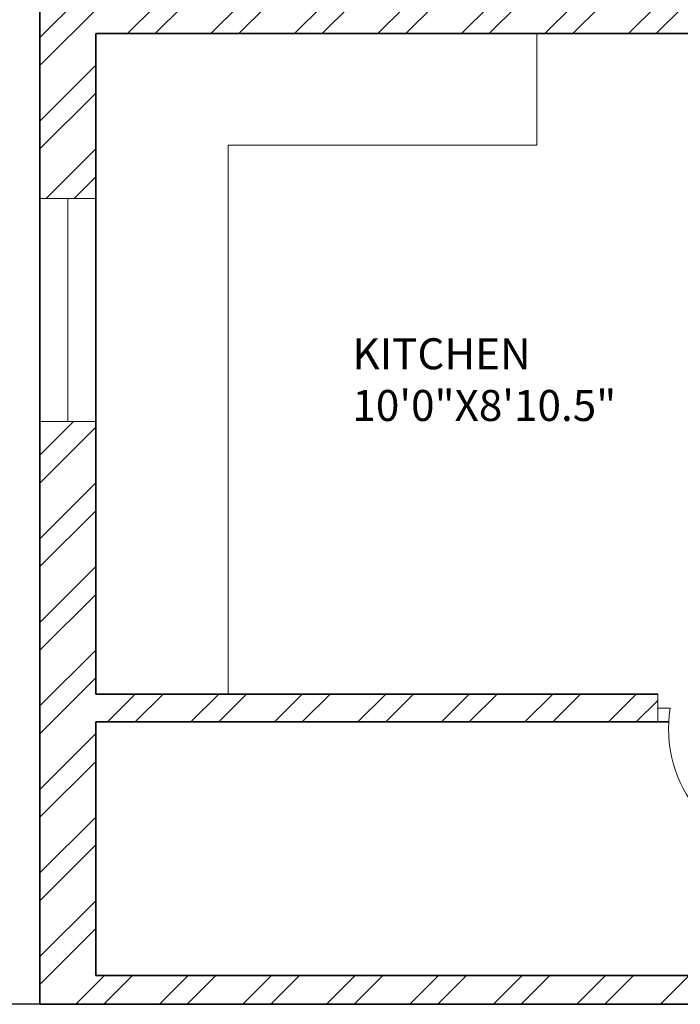
# Model space of a CAD drawing. Units: inches. Extents: x 2120 to 4013, y 1390 to 3019.
# Tile 2 of 59: x 2259 to 2366, y 1582 to 1740. Entities that reach past the tile are written whole.
import ezdxf

# ---------------------------------------------------------------- set-up
doc = ezdxf.new("R2010")
doc.units = ezdxf.units.IN
for name, color, linetype, lineweight in [('A-ANNO-DIMS', 2, 'Continuous', 18), ('A-AREA-IDEN', 7, 'Continuous', 18), ('A-DOOR', 3, 'Continuous', 18), ('A-FLOR-CASE', 8, 'Continuous', 18), ('A-GLAZ', 4, 'Continuous', 18), ('A-WALL', 7, 'Continuous', 35), ('A-WALL-PATT', 252, 'Continuous', 13)]:
    doc.layers.add(name, color=color, linetype=linetype, lineweight=lineweight)
doc.styles.get("Standard").update_dxf_attribs({"font": 'arial.ttf'})
doc.dimstyles.get("Standard").update_dxf_attribs({"dimtxt": 0.18, "dimasz": 0.18, "dimexe": 0.18, "dimexo": 0.0625, "dimgap": 0.09, "dimtad": 0, "dimtih": 1, "dimtoh": 1, "dimdec": 4, "dimzin": 0, "dimdsep": 46, "dimtxsty": 'Standard', "dimcen": 0.09, "dimadec": 0, "dimazin": 0, "dimtfac": 1, "dimtdec": 4, "dimtofl": 0, "dimtmove": 0, "dimatfit": 3, "dimfxl": 1, "dimtolj": 1, "dimtzin": 0, "dimarcsym": 0})

# ---------------------------------------------------------------- blocks, each defined once
blk = doc.blocks.new('DOOR-SWING-24IN-99p42DEG')
for p, q in [((0, 26.25), (0, 21.75)), ((24.35, 21.75), (24.35, 26.25)), ((24.35, 26.25), (24.35, 24)), ((0, 21.75), (0, 24)), ((0, 24), (2, 24)), ((24.35, 24), (22.35, 24)), ((22.35, 24), (22.35, 0))]:
    blk.add_line(p, q)
blk.add_arc((22.35, 20.62), 20.62, 170.5813, 270)
blk = doc.blocks.new('WIN-PLAN-36IN-03')
for p, q in [((9, 36), (0, 36)), ((0, 36), (4.5, 36)), ((4.5, 36), (4.5, 0)), ((9, 0), (0, 0)), ((4.5, 0), (9, 0))]:
    blk.add_line(p, q)
blk = doc.blocks.new('*D213')
at = {"layer": 'A-ANNO-DIMS', "color": 0, "lineweight": -2, "transparency": 16777216}
for p, q in [((2271.67, 1865.53), (2217.55, 1865.53)), ((2217.73, 1865.35), (2217.73, 1723.71)), ((2217.73, 1581.71), (2217.73, 1723.35)), ((2262.67, 1581.53), (2217.55, 1581.53))]:
    blk.add_line(p, q, dxfattribs=at)
at = {"layer": 'A-ANNO-DIMS', "color": 0, "transparency": 16777216}
for points in [[(2217.7, 1865.35), (2217.76, 1865.35), (2217.73, 1865.53)], [(2217.7, 1581.71), (2217.76, 1581.71), (2217.73, 1581.53)]]:
    blk.add_solid(points, dxfattribs=at)
at = {"layer": 'Defpoints', "color": 0, "transparency": 16777216}
for p in [(2217.73, 1865.53), (2271.73, 1865.53), (2262.73, 1581.53)]:
    blk.add_point(p, dxfattribs=at)
at = {"layer": 'A-ANNO-DIMS', "color": 0, "transparency": 16777216, "insert": (2217.73, 1723.53), "char_height": 0.18, "attachment_point": 5}
blk.add_mtext('\\A1;284', dxfattribs=at)

msp = doc.modelspace()

# ---------------------------------------------------------------- hatches: boundary and pattern name
at = {"layer": 'A-WALL-PATT'}
h = msp.add_hatch(dxfattribs=at)
h.set_pattern_fill('ANSI32', color=256)
h.paths.add_polyline_path([(2271.7331, 2343.531), (2283.3788, 2343.531), (2283.3788, 2348.031), (2283.3788, 2352.5306), (2262.7331, 2352.5306), (2262.7331, 2182.638), (2267.2331, 2182.638), (2271.7331, 2182.638), (2271.7331, 2219.031), (2391.7331, 2219.031), (2391.7331, 2214.189), (2393.9831, 2214.189), (2396.2331, 2214.189), (2396.2331, 2219.031), (2420.2331, 2219.031), (2420.2331, 2225.7535), (2417.2197, 2225.7535), (2415.7331, 2225.7535), (2415.7331, 2223.5306), (2271.7331, 2223.5306)])
h.paths.add_polyline_path([(2380.0942, 2352.5306), (2343.3788, 2352.5306), (2343.3788, 2343.531), (2363.2331, 2343.531), (2363.2331, 2288.8489), (2365.4831, 2288.8489), (2367.7331, 2288.8489), (2367.7331, 2343.531), (2380.0942, 2343.531)], flags=17)
h.paths.add_polyline_path([(2432.4339, 2352.5306), (2404.0943, 2352.5306), (2404.0943, 2343.531), (2415.7331, 2343.531), (2415.7331, 2264.0306), (2367.7331, 2264.0306), (2367.7331, 2266.4872), (2363.2331, 2266.4872), (2363.2331, 2259.531), (2367.7331, 2259.531), (2415.7331, 2259.531), (2415.7331, 2255.0658), (2420.2331, 2255.0658), (2420.2331, 2259.531), (2424.5717, 2259.531), (2424.5717, 2261.781), (2424.5717, 2264.0306), (2420.2331, 2264.0306), (2420.2331, 2343.531), (2432.4339, 2343.531)])
h.paths.add_polyline_path([(2508.9115, 2352.5306), (2456.4339, 2352.5306), (2456.4339, 2343.531), (2468.2331, 2343.531), (2468.2331, 2264.0306), (2448.0487, 2264.0306), (2448.0487, 2259.531), (2468.2331, 2259.531), (2468.2331, 2255.5496), (2472.7331, 2255.5496), (2472.7331, 2343.531), (2508.9115, 2343.531)])
h.paths.add_polyline_path([(2637.7331, 2352.5306), (2544.9116, 2352.5306), (2544.9116, 2343.531), (2589.7331, 2343.531), (2633.2331, 2343.531), (2637.7331, 2343.531)])
h.paths.add_polyline_path([(2594.2331, 2343.5306), (2589.7331, 2343.5306), (2589.7331, 2259.5306), (2589.7331, 2252.4915), (2591.9831, 2252.4915), (2594.2331, 2252.4915)])
h.paths.add_polyline_path([(2637.7331, 2223.5306), (2594.2331, 2223.5306), (2594.2331, 2230.1988), (2591.9831, 2230.1988), (2589.7331, 2230.1988), (2589.7331, 2223.5306), (2472.7331, 2223.5306), (2468.2331, 2223.5306), (2468.2331, 2219.031), (2628.7331, 2219.031), (2628.7331, 2138.031), (2637.7331, 2138.031)])
h.paths.add_polyline_path([(3822.6535, 2458.4402), (3874.9468, 2458.4402), (3874.9468, 2476.9866), (3822.6535, 2476.9866)], flags=9)
h.paths.add_polyline_path([(3834.6921, 2781.8174), (3935.9206, 2781.8174), (3935.9206, 2800.3638), (3834.6921, 2800.3638)], flags=9)
h.paths.add_polyline_path([(3832.2843, 2837.9683), (3884.5776, 2837.9683), (3884.5776, 2856.5146), (3832.2843, 2856.5146)], flags=9)
h.paths.add_polyline_path([(3830.9388, 2861.4782), (3956.8958, 2861.4782), (3956.8958, 2880.0245), (3830.9388, 2880.0245)], flags=9)
h.paths.add_polyline_path([(3870.6966, 2352.5752), (3887.9272, 2352.5752), (3887.9272, 2377.3037), (3870.6966, 2377.3037)], flags=9)
h.paths.add_polyline_path([(3289.2701, 2413.161), (3435.2223, 2413.161), (3435.2223, 2450.2538), (3289.2701, 2450.2538)], flags=9)
h.paths.add_polyline_path([(2487.6944, 2414.3601), (2637.8335, 2414.3601), (2637.8335, 2451.4528), (2487.6944, 2451.4528)], flags=9)
h.paths.add_polyline_path([(2567.3724, 1457.9199), (2815.296, 1457.9199), (2815.296, 1495.0127), (2567.3724, 1495.0127)], flags=9)
h.paths.add_polyline_path([(2655.3825, 2093.2363), (2685.9555, 2093.2363), (2685.9555, 2111.8937), (2655.3825, 2111.8937)], flags=9)
h.paths.add_polyline_path([(2543.9218, 1550.6671), (2587.8406, 1550.6671), (2587.8406, 1569.3244), (2543.9218, 1569.3244)], flags=9)
h.paths.add_polyline_path([(2905.1384, 1543.8113), (2949.0572, 1543.8113), (2949.0572, 1562.4686), (2905.1384, 1562.4686)], flags=9)
h.paths.add_polyline_path([(2736.4118, 1702.4736), (2784.2153, 1702.4736), (2784.2153, 1721.1309), (2736.4118, 1721.1309)], flags=9)
h.paths.add_polyline_path([(2912.8666, 1710.4168), (2951.707, 1710.4168), (2951.707, 1729.0741), (2912.8666, 1729.0741)], flags=9)
h.paths.add_polyline_path([(2923.5785, 1763.5038), (2959.7279, 1763.5038), (2959.7279, 1782.1611), (2923.5785, 1782.1611)], flags=9)
h.paths.add_polyline_path([(2925.2114, 1809.6137), (2967.1861, 1809.6137), (2967.1861, 1828.271), (2925.2114, 1828.271)], flags=9)
h.paths.add_polyline_path([(2996.2711, 1878.9003), (2996.2711, 1913.109), (2977.6138, 1913.109), (2977.6138, 1878.9003)], flags=9)
h.paths.add_polyline_path([(2883.0859, 1895.7192), (2927.1855, 1895.7192), (2927.1855, 1914.3766), (2883.0859, 1914.3766)], flags=9)
h.paths.add_polyline_path([(2787.3924, 1810.8013), (2841.0213, 1810.8013), (2841.0213, 1829.4587), (2787.3924, 1829.4587)], flags=9)
h.paths.add_polyline_path([(2775.6399, 2101.7395), (2829.2689, 2101.7395), (2829.2689, 2120.3968), (2775.6399, 2120.3968)], flags=9)
h.paths.add_polyline_path([(2913.0263, 2075.817), (2951.8667, 2075.817), (2951.8667, 2094.4744), (2913.0263, 2094.4744)], flags=9)
h.paths.add_polyline_path([(2929.966, 2133.3669), (2966.1154, 2133.3669), (2966.1154, 2152.0243), (2929.966, 2152.0243)], flags=9)
h.paths.add_polyline_path([(2932.7502, 2182.6088), (2968.8996, 2182.6088), (2968.8996, 2201.2662), (2932.7502, 2201.2662)], flags=9)
h.paths.add_polyline_path([(2996.0681, 2266.3173), (2996.0681, 2300.5261), (2977.4108, 2300.5261), (2977.4108, 2266.3173)], flags=9)
h.paths.add_polyline_path([(2885.1039, 2279.2186), (2929.2035, 2279.2186), (2929.2035, 2297.8759), (2885.1039, 2297.8759)], flags=9)
h.paths.add_polyline_path([(2735.7042, 2218.3197), (2783.5078, 2218.3197), (2783.5078, 2236.9771), (2735.7042, 2236.9771)], flags=9)
h.paths.add_polyline_path([(2635.6049, 2044.0085), (2648.9678, 2044.0085), (2648.9678, 2054.312), (2635.6049, 2054.312)], flags=9)
h.paths.add_polyline_path([(2714.0148, 1923.0473), (2727.3777, 1923.0473), (2727.3777, 1933.3508), (2714.0148, 1933.3508)], flags=9)
h.paths.add_polyline_path([(2709.0345, 1988.1628), (2722.3974, 1988.1628), (2722.3974, 1998.4663), (2709.0345, 1998.4663)], flags=9)
h.paths.add_polyline_path([(2592.8935, 1962.1763), (2606.2564, 1962.1763), (2606.2564, 1972.4799), (2592.8935, 1972.4799)], flags=9)
h.paths.add_polyline_path([(2618.3996, 1985.9724), (2644.1942, 1985.9724), (2644.1942, 1996.2759), (2618.3996, 1996.2759)], flags=9)
h.paths.add_polyline_path([(2601.279, 1920.5869), (2614.6419, 1920.5869), (2614.6419, 1930.8904), (2601.279, 1930.8904)], flags=9)
h.paths.add_polyline_path([(2692.3278, 1932.7645), (2704.5311, 1932.7645), (2704.5311, 1943.0681), (2692.3278, 1943.0681)], flags=9)
h.paths.add_polyline_path([(2311.122, 1672.7318), (2355.0408, 1672.7318), (2355.0408, 1691.3892), (2311.122, 1691.3892)], flags=9)
h.paths.add_polyline_path([(2456.2551, 1632.3198), (2492.4796, 1632.3198), (2492.4796, 1650.9772), (2456.2551, 1650.9772)], flags=9)
h.paths.add_polyline_path([(2401.0766, 1631.4793), (2437.301, 1631.4793), (2437.301, 1650.1367), (2401.0766, 1650.1367)], flags=9)
h.paths.add_polyline_path([(2546.7054, 1700.9235), (2594.509, 1700.9235), (2594.509, 1719.5809), (2546.7054, 1719.5809)], flags=9)
h.paths.add_polyline_path([(2445.4866, 1766.9937), (2497.5261, 1766.9937), (2497.5261, 1785.651), (2445.4866, 1785.651)], flags=9)
h.paths.add_polyline_path([(2287.9992, 1739.7675), (2326.8396, 1739.7675), (2326.8396, 1758.4248), (2287.9992, 1758.4248)], flags=9)
h.paths.add_polyline_path([(2458.5279, 1924.7607), (2510.5675, 1924.7607), (2510.5675, 1943.4181), (2458.5279, 1943.4181)], flags=9)
h.paths.add_polyline_path([(2309.2811, 1902.7642), (2345.4305, 1902.7642), (2345.4305, 1921.4215), (2309.2811, 1921.4215)], flags=9)
h.paths.add_polyline_path([(2490.7554, 2018.9392), (2530.7896, 2018.9392), (2530.7896, 2037.5965), (2490.7554, 2037.5965)], flags=9)
h.paths.add_polyline_path([(2402.143, 2024.7393), (2438.5414, 2024.7393), (2438.5414, 2043.3966), (2402.143, 2043.3966)], flags=9)
h.paths.add_polyline_path([(2287.856, 1931.7926), (2326.6964, 1931.7926), (2326.6964, 1950.4499), (2287.856, 1950.4499)], flags=9)
h.paths.add_polyline_path([(2281.7979, 2193.5771), (2320.6383, 2193.5771), (2320.6383, 2212.2344), (2281.7979, 2212.2344)], flags=25)
h.paths.add_polyline_path([(2484.0754, 2093.892), (2536.115, 2093.892), (2536.115, 2112.5494), (2484.0754, 2112.5494)], flags=9)
h.paths.add_polyline_path([(2624.7948, 2281.8639), (2624.7948, 2311.4137), (2606.1375, 2311.4137), (2606.1375, 2281.8639)], flags=9)
h.paths.add_polyline_path([(2507.5036, 2290.3639), (2541.934, 2290.3639), (2541.934, 2309.0212), (2507.5036, 2309.0212)], flags=9)
h.paths.add_polyline_path([(2423.1076, 2285.2202), (2459.332, 2285.2202), (2459.332, 2303.8776), (2423.1076, 2303.8776)], flags=9)
h.paths.add_polyline_path([(2374.5467, 2289.6272), (2410.7711, 2289.6272), (2410.7711, 2308.2846), (2374.5467, 2308.2846)], flags=25)
h.paths.add_polyline_path([(2277.4907, 2227.5651), (2316.3311, 2227.5651), (2316.3311, 2246.2224), (2277.4907, 2246.2224)], flags=25)
h.paths.add_polyline_path([(2655.3825, 2093.2367), (2685.9555, 2093.2367), (2685.9555, 2111.894), (2655.3825, 2111.894)], flags=9)
h.paths.add_polyline_path([(2543.9217, 1550.6674), (2587.8406, 1550.6674), (2587.8406, 1569.3247), (2543.9217, 1569.3247)], flags=9)
h.paths.add_polyline_path([(2905.1384, 1543.8116), (2949.0572, 1543.8116), (2949.0572, 1562.4689), (2905.1384, 1562.4689)], flags=9)
h.paths.add_polyline_path([(2736.4118, 1702.4739), (2784.2153, 1702.4739), (2784.2153, 1721.1312), (2736.4118, 1721.1312)], flags=9)
h.paths.add_polyline_path([(2912.8666, 1710.4171), (2951.707, 1710.4171), (2951.707, 1729.0744), (2912.8666, 1729.0744)], flags=9)
h.paths.add_polyline_path([(2923.5785, 1763.5041), (2959.7279, 1763.5041), (2959.7279, 1782.1614), (2923.5785, 1782.1614)], flags=9)
h.paths.add_polyline_path([(2925.2114, 1809.614), (2967.1861, 1809.614), (2967.1861, 1828.2713), (2925.2114, 1828.2713)], flags=9)
h.paths.add_polyline_path([(2996.2711, 1878.9006), (2996.2711, 1913.1094), (2977.6137, 1913.1094), (2977.6137, 1878.9006)], flags=9)
h.paths.add_polyline_path([(2883.0859, 1895.7195), (2927.1855, 1895.7195), (2927.1855, 1914.3769), (2883.0859, 1914.3769)], flags=9)
h.paths.add_polyline_path([(2787.3924, 1810.8016), (2841.0213, 1810.8016), (2841.0213, 1829.459), (2787.3924, 1829.459)], flags=9)
h.paths.add_polyline_path([(2775.6399, 2101.7398), (2829.2688, 2101.7398), (2829.2688, 2120.3971), (2775.6399, 2120.3971)], flags=9)
h.paths.add_polyline_path([(2913.0263, 2075.8173), (2951.8667, 2075.8173), (2951.8667, 2094.4747), (2913.0263, 2094.4747)], flags=9)
h.paths.add_polyline_path([(2929.966, 2133.3672), (2966.1154, 2133.3672), (2966.1154, 2152.0246), (2929.966, 2152.0246)], flags=9)
h.paths.add_polyline_path([(2932.7502, 2182.6091), (2968.8996, 2182.6091), (2968.8996, 2201.2665), (2932.7502, 2201.2665)], flags=9)
h.paths.add_polyline_path([(2996.0681, 2266.3176), (2996.0681, 2300.5264), (2977.4108, 2300.5264), (2977.4108, 2266.3176)], flags=9)
h.paths.add_polyline_path([(2885.1039, 2279.2189), (2929.2035, 2279.2189), (2929.2035, 2297.8762), (2885.1039, 2297.8762)], flags=9)
h.paths.add_polyline_path([(2735.7042, 2218.32), (2783.5078, 2218.32), (2783.5078, 2236.9774), (2735.7042, 2236.9774)], flags=9)
h.paths.add_polyline_path([(2635.6048, 2044.0088), (2648.9677, 2044.0088), (2648.9677, 2054.3123), (2635.6048, 2054.3123)], flags=9)
h.paths.add_polyline_path([(2714.0148, 1923.0476), (2727.3777, 1923.0476), (2727.3777, 1933.3511), (2714.0148, 1933.3511)], flags=9)
h.paths.add_polyline_path([(2709.0345, 1988.1631), (2722.3974, 1988.1631), (2722.3974, 1998.4666), (2709.0345, 1998.4666)], flags=9)
h.paths.add_polyline_path([(2592.8935, 1962.1766), (2606.2564, 1962.1766), (2606.2564, 1972.4802), (2592.8935, 1972.4802)], flags=9)
h.paths.add_polyline_path([(2618.3995, 1985.9727), (2644.1942, 1985.9727), (2644.1942, 1996.2762), (2618.3995, 1996.2762)], flags=9)
h.paths.add_polyline_path([(2601.279, 1920.5872), (2614.6419, 1920.5872), (2614.6419, 1930.8908), (2601.279, 1930.8908)], flags=9)
h.paths.add_polyline_path([(2692.3278, 1932.7648), (2704.5311, 1932.7648), (2704.5311, 1943.0684), (2692.3278, 1943.0684)], flags=9)
h.paths.add_polyline_path([(2311.122, 1672.7321), (2355.0408, 1672.7321), (2355.0408, 1691.3895), (2311.122, 1691.3895)], flags=9)
h.paths.add_polyline_path([(2456.2551, 1632.3201), (2492.4795, 1632.3201), (2492.4795, 1650.9775), (2456.2551, 1650.9775)], flags=9)
h.paths.add_polyline_path([(2401.0766, 1631.4796), (2437.301, 1631.4796), (2437.301, 1650.137), (2401.0766, 1650.137)], flags=9)
h.paths.add_polyline_path([(2546.7054, 1700.9238), (2594.509, 1700.9238), (2594.509, 1719.5812), (2546.7054, 1719.5812)], flags=9)
h.paths.add_polyline_path([(2445.4866, 1766.994), (2497.5261, 1766.994), (2497.5261, 1785.6513), (2445.4866, 1785.6513)], flags=9)
h.paths.add_polyline_path([(2287.9992, 1739.7678), (2326.8396, 1739.7678), (2326.8396, 1758.4251), (2287.9992, 1758.4251)], flags=9)
h.paths.add_polyline_path([(2458.5279, 1924.7611), (2510.5675, 1924.7611), (2510.5675, 1943.4184), (2458.5279, 1943.4184)], flags=9)
h.paths.add_polyline_path([(2309.2811, 1902.7645), (2345.4305, 1902.7645), (2345.4305, 1921.4218), (2309.2811, 1921.4218)], flags=9)
h.paths.add_polyline_path([(2490.7554, 2018.9395), (2530.7895, 2018.9395), (2530.7895, 2037.5968), (2490.7554, 2037.5968)], flags=9)
h.paths.add_polyline_path([(2402.143, 2024.7396), (2438.5413, 2024.7396), (2438.5413, 2043.3969), (2402.143, 2043.3969)], flags=9)
h.paths.add_polyline_path([(2287.856, 1931.7929), (2326.6964, 1931.7929), (2326.6964, 1950.4502), (2287.856, 1950.4502)], flags=9)
h.paths.add_polyline_path([(2281.7979, 2193.5774), (2320.6383, 2193.5774), (2320.6383, 2212.2347), (2281.7979, 2212.2347)], flags=25)
h.paths.add_polyline_path([(2484.0754, 2093.8924), (2536.115, 2093.8924), (2536.115, 2112.5497), (2484.0754, 2112.5497)], flags=9)
h.paths.add_polyline_path([(2624.7948, 2281.8642), (2624.7948, 2311.414), (2606.1374, 2311.414), (2606.1374, 2281.8642)], flags=9)
h.paths.add_polyline_path([(2507.5035, 2290.3642), (2541.934, 2290.3642), (2541.934, 2309.0215), (2507.5035, 2309.0215)], flags=9)
h.paths.add_polyline_path([(2423.1075, 2285.2205), (2459.332, 2285.2205), (2459.332, 2303.8779), (2423.1075, 2303.8779)], flags=9)
h.paths.add_polyline_path([(2374.5467, 2289.6275), (2410.7711, 2289.6275), (2410.7711, 2308.2849), (2374.5467, 2308.2849)], flags=25)
h.paths.add_polyline_path([(2277.4907, 2227.5654), (2316.3311, 2227.5654), (2316.3311, 2246.2227), (2277.4907, 2246.2227)], flags=25)
h = msp.add_hatch(dxfattribs=at)
h.set_pattern_fill('ANSI32', color=256)
h.paths.add_polyline_path([(2271.7331, 1980.389), (2262.7331, 1980.389), (2262.7331, 1912.8434), (2267.2331, 1912.8434), (2271.7331, 1912.8434), (2271.7331, 1922.531), (2351.2331, 1922.531), (2351.2331, 1901.4728), (2355.7331, 1901.4728), (2355.7331, 1922.531), (2357.9815, 1922.531), (2357.9815, 1926.5306), (2271.7331, 1926.5306)])
h.paths.add_polyline_path([(2589.2331, 1949.1622), (2584.7331, 1949.1622), (2580.2331, 1949.1622), (2580.2331, 1874.5306), (2355.7331, 1874.5306), (2355.7331, 1880.1922), (2351.2331, 1880.1922), (2351.2331, 1874.5306), (2271.7331, 1874.5306), (2271.7331, 1888.8431), (2262.7331, 1888.8431), (2262.7331, 1842.2909), (2267.2331, 1842.2909), (2271.7331, 1842.2909), (2271.7331, 1865.531), (2415.7331, 1865.531), (2415.7331, 1779.7286), (2420.2331, 1779.7286), (2420.2331, 1865.531), (2589.2331, 1865.531)])
h.paths.add_polyline_path([(2271.7331, 1782.2906), (2262.7331, 1782.2906), (2262.7331, 1711.4639), (2267.2331, 1711.4639), (2271.7331, 1711.4639), (2271.7331, 1738.031), (2420.2331, 1738.031), (2420.2331, 1742.531), (2420.2331, 1747.3376), (2417.9831, 1747.3376), (2415.7331, 1747.3376), (2415.7331, 1742.5306), (2271.7331, 1742.5306)])
h.paths.add_polyline_path([(2271.7331, 1627.031), (2362.3957, 1627.031), (2362.3957, 1629.281), (2362.3957, 1631.5306), (2271.7331, 1631.5306), (2271.7331, 1675.4636), (2262.7331, 1675.4636), (2262.7331, 1581.531), (2405.3032, 1581.531), (2405.3032, 1586.031), (2405.3032, 1590.5306), (2396.2331, 1590.5306), (2396.2331, 1691.4513), (2418.7206, 1691.4513), (2418.7206, 1695.951), (2396.2331, 1695.951), (2391.7331, 1695.951), (2391.7331, 1631.5306), (2386.7425, 1631.5306), (2386.7425, 1629.2806), (2386.7425, 1627.031), (2391.7331, 1627.031), (2391.7331, 1586.1709), (2271.7331, 1586.1709)])
h.paths.add_polyline_path([(2459.6703, 1590.5306), (2429.3032, 1590.5306), (2429.3032, 1581.531), (2459.6703, 1581.531), (2459.6703, 1586.031)])
h.paths.add_polyline_path([(2501.2331, 1590.531), (2501.2331, 1665.0195), (2498.9831, 1665.0195), (2496.7331, 1665.0195), (2496.7331, 1590.5306), (2483.8201, 1590.5306), (2483.8201, 1590.1579), (2483.6704, 1590.1579), (2483.6704, 1581.531), (2505.0196, 1581.531), (2505.0196, 1583.781), (2505.0196, 1586.0306), (2501.2331, 1586.0306)])
h.paths.add_polyline_path([(2544.1361, 1583.781), (2544.1361, 1586.0306), (2527.1368, 1586.0306), (2527.1368, 1583.7806), (2527.1368, 1581.531), (2544.1361, 1581.531)])
h.paths.add_polyline_path([(3822.6535, 2458.4402), (3874.9468, 2458.4402), (3874.9468, 2476.9866), (3822.6535, 2476.9866)], flags=9)
h.paths.add_polyline_path([(3834.6921, 2781.8174), (3935.9206, 2781.8174), (3935.9206, 2800.3638), (3834.6921, 2800.3638)], flags=9)
h.paths.add_polyline_path([(3832.2843, 2837.9683), (3884.5776, 2837.9683), (3884.5776, 2856.5146), (3832.2843, 2856.5146)], flags=9)
h.paths.add_polyline_path([(3830.9388, 2861.4782), (3956.8958, 2861.4782), (3956.8958, 2880.0245), (3830.9388, 2880.0245)], flags=9)
h.paths.add_polyline_path([(3870.6966, 2352.5752), (3887.9272, 2352.5752), (3887.9272, 2377.3037), (3870.6966, 2377.3037)], flags=9)
h.paths.add_polyline_path([(3289.2701, 2413.161), (3435.2223, 2413.161), (3435.2223, 2450.2538), (3289.2701, 2450.2538)], flags=9)
h.paths.add_polyline_path([(2487.6944, 2414.3601), (2637.8335, 2414.3601), (2637.8335, 2451.4528), (2487.6944, 2451.4528)], flags=9)
h.paths.add_polyline_path([(2567.3724, 1457.9199), (2815.296, 1457.9199), (2815.296, 1495.0127), (2567.3724, 1495.0127)], flags=9)
h.paths.add_polyline_path([(2655.3825, 2093.2363), (2685.9555, 2093.2363), (2685.9555, 2111.8937), (2655.3825, 2111.8937)], flags=9)
h.paths.add_polyline_path([(2543.9218, 1550.6671), (2587.8406, 1550.6671), (2587.8406, 1569.3244), (2543.9218, 1569.3244)], flags=9)
h.paths.add_polyline_path([(2905.1384, 1543.8113), (2949.0572, 1543.8113), (2949.0572, 1562.4686), (2905.1384, 1562.4686)], flags=9)
h.paths.add_polyline_path([(2736.4118, 1702.4736), (2784.2153, 1702.4736), (2784.2153, 1721.1309), (2736.4118, 1721.1309)], flags=9)
h.paths.add_polyline_path([(2912.8666, 1710.4168), (2951.707, 1710.4168), (2951.707, 1729.0741), (2912.8666, 1729.0741)], flags=9)
h.paths.add_polyline_path([(2923.5785, 1763.5038), (2959.7279, 1763.5038), (2959.7279, 1782.1611), (2923.5785, 1782.1611)], flags=9)
h.paths.add_polyline_path([(2925.2114, 1809.6137), (2967.1861, 1809.6137), (2967.1861, 1828.271), (2925.2114, 1828.271)], flags=9)
h.paths.add_polyline_path([(2996.2711, 1878.9003), (2996.2711, 1913.109), (2977.6138, 1913.109), (2977.6138, 1878.9003)], flags=9)
h.paths.add_polyline_path([(2883.0859, 1895.7192), (2927.1855, 1895.7192), (2927.1855, 1914.3766), (2883.0859, 1914.3766)], flags=9)
h.paths.add_polyline_path([(2787.3924, 1810.8013), (2841.0213, 1810.8013), (2841.0213, 1829.4587), (2787.3924, 1829.4587)], flags=9)
h.paths.add_polyline_path([(2775.6399, 2101.7395), (2829.2689, 2101.7395), (2829.2689, 2120.3968), (2775.6399, 2120.3968)], flags=9)
h.paths.add_polyline_path([(2913.0263, 2075.817), (2951.8667, 2075.817), (2951.8667, 2094.4744), (2913.0263, 2094.4744)], flags=9)
h.paths.add_polyline_path([(2929.966, 2133.3669), (2966.1154, 2133.3669), (2966.1154, 2152.0243), (2929.966, 2152.0243)], flags=9)
h.paths.add_polyline_path([(2932.7502, 2182.6088), (2968.8996, 2182.6088), (2968.8996, 2201.2662), (2932.7502, 2201.2662)], flags=9)
h.paths.add_polyline_path([(2996.0681, 2266.3173), (2996.0681, 2300.5261), (2977.4108, 2300.5261), (2977.4108, 2266.3173)], flags=9)
h.paths.add_polyline_path([(2885.1039, 2279.2186), (2929.2035, 2279.2186), (2929.2035, 2297.8759), (2885.1039, 2297.8759)], flags=9)
h.paths.add_polyline_path([(2735.7042, 2218.3197), (2783.5078, 2218.3197), (2783.5078, 2236.9771), (2735.7042, 2236.9771)], flags=9)
h.paths.add_polyline_path([(2635.6049, 2044.0085), (2648.9678, 2044.0085), (2648.9678, 2054.312), (2635.6049, 2054.312)], flags=9)
h.paths.add_polyline_path([(2714.0148, 1923.0473), (2727.3777, 1923.0473), (2727.3777, 1933.3508), (2714.0148, 1933.3508)], flags=9)
h.paths.add_polyline_path([(2709.0345, 1988.1628), (2722.3974, 1988.1628), (2722.3974, 1998.4663), (2709.0345, 1998.4663)], flags=9)
h.paths.add_polyline_path([(2592.8935, 1962.1763), (2606.2564, 1962.1763), (2606.2564, 1972.4799), (2592.8935, 1972.4799)], flags=9)
h.paths.add_polyline_path([(2618.3996, 1985.9724), (2644.1942, 1985.9724), (2644.1942, 1996.2759), (2618.3996, 1996.2759)], flags=9)
h.paths.add_polyline_path([(2601.279, 1920.5869), (2614.6419, 1920.5869), (2614.6419, 1930.8904), (2601.279, 1930.8904)], flags=9)
h.paths.add_polyline_path([(2692.3278, 1932.7645), (2704.5311, 1932.7645), (2704.5311, 1943.0681), (2692.3278, 1943.0681)], flags=9)
h.paths.add_polyline_path([(2311.122, 1672.7318), (2355.0408, 1672.7318), (2355.0408, 1691.3892), (2311.122, 1691.3892)], flags=25)
h.paths.add_polyline_path([(2456.2551, 1632.3198), (2492.4796, 1632.3198), (2492.4796, 1650.9772), (2456.2551, 1650.9772)], flags=9)
h.paths.add_polyline_path([(2401.0766, 1631.4793), (2437.301, 1631.4793), (2437.301, 1650.1367), (2401.0766, 1650.1367)], flags=9)
h.paths.add_polyline_path([(2546.7054, 1700.9235), (2594.509, 1700.9235), (2594.509, 1719.5809), (2546.7054, 1719.5809)], flags=9)
h.paths.add_polyline_path([(2445.4866, 1766.9937), (2497.5261, 1766.9937), (2497.5261, 1785.651), (2445.4866, 1785.651)], flags=9)
h.paths.add_polyline_path([(2287.9992, 1739.7675), (2326.8396, 1739.7675), (2326.8396, 1758.4248), (2287.9992, 1758.4248)], flags=24)
h.paths.add_polyline_path([(2458.5279, 1924.7607), (2510.5675, 1924.7607), (2510.5675, 1943.4181), (2458.5279, 1943.4181)], flags=25)
h.paths.add_polyline_path([(2309.2811, 1902.7642), (2345.4305, 1902.7642), (2345.4305, 1921.4215), (2309.2811, 1921.4215)], flags=25)
h.paths.add_polyline_path([(2490.7554, 2018.9392), (2530.7896, 2018.9392), (2530.7896, 2037.5965), (2490.7554, 2037.5965)], flags=9)
h.paths.add_polyline_path([(2402.143, 2024.7393), (2438.5414, 2024.7393), (2438.5414, 2043.3966), (2402.143, 2043.3966)], flags=9)
h.paths.add_polyline_path([(2287.856, 1931.7926), (2326.6964, 1931.7926), (2326.6964, 1950.4499), (2287.856, 1950.4499)], flags=25)
h.paths.add_polyline_path([(2281.7979, 2193.5771), (2320.6383, 2193.5771), (2320.6383, 2212.2344), (2281.7979, 2212.2344)], flags=9)
h.paths.add_polyline_path([(2484.0754, 2093.892), (2536.115, 2093.892), (2536.115, 2112.5494), (2484.0754, 2112.5494)], flags=9)
h.paths.add_polyline_path([(2624.7948, 2281.8639), (2624.7948, 2311.4137), (2606.1375, 2311.4137), (2606.1375, 2281.8639)], flags=9)
h.paths.add_polyline_path([(2507.5036, 2290.3639), (2541.934, 2290.3639), (2541.934, 2309.0212), (2507.5036, 2309.0212)], flags=9)
h.paths.add_polyline_path([(2423.1076, 2285.2202), (2459.332, 2285.2202), (2459.332, 2303.8776), (2423.1076, 2303.8776)], flags=9)
h.paths.add_polyline_path([(2374.5467, 2289.6272), (2410.7711, 2289.6272), (2410.7711, 2308.2846), (2374.5467, 2308.2846)], flags=9)
h.paths.add_polyline_path([(2277.4907, 2227.5651), (2316.3311, 2227.5651), (2316.3311, 2246.2224), (2277.4907, 2246.2224)], flags=9)
h.paths.add_polyline_path([(2655.3825, 2093.2367), (2685.9555, 2093.2367), (2685.9555, 2111.894), (2655.3825, 2111.894)], flags=9)
h.paths.add_polyline_path([(2543.9217, 1550.6674), (2587.8406, 1550.6674), (2587.8406, 1569.3247), (2543.9217, 1569.3247)], flags=9)
h.paths.add_polyline_path([(2905.1384, 1543.8116), (2949.0572, 1543.8116), (2949.0572, 1562.4689), (2905.1384, 1562.4689)], flags=9)
h.paths.add_polyline_path([(2736.4118, 1702.4739), (2784.2153, 1702.4739), (2784.2153, 1721.1312), (2736.4118, 1721.1312)], flags=9)
h.paths.add_polyline_path([(2912.8666, 1710.4171), (2951.707, 1710.4171), (2951.707, 1729.0744), (2912.8666, 1729.0744)], flags=9)
h.paths.add_polyline_path([(2923.5785, 1763.5041), (2959.7279, 1763.5041), (2959.7279, 1782.1614), (2923.5785, 1782.1614)], flags=9)
h.paths.add_polyline_path([(2925.2114, 1809.614), (2967.1861, 1809.614), (2967.1861, 1828.2713), (2925.2114, 1828.2713)], flags=9)
h.paths.add_polyline_path([(2996.2711, 1878.9006), (2996.2711, 1913.1094), (2977.6137, 1913.1094), (2977.6137, 1878.9006)], flags=9)
h.paths.add_polyline_path([(2883.0859, 1895.7195), (2927.1855, 1895.7195), (2927.1855, 1914.3769), (2883.0859, 1914.3769)], flags=9)
h.paths.add_polyline_path([(2787.3924, 1810.8016), (2841.0213, 1810.8016), (2841.0213, 1829.459), (2787.3924, 1829.459)], flags=9)
h.paths.add_polyline_path([(2775.6399, 2101.7398), (2829.2688, 2101.7398), (2829.2688, 2120.3971), (2775.6399, 2120.3971)], flags=9)
h.paths.add_polyline_path([(2913.0263, 2075.8173), (2951.8667, 2075.8173), (2951.8667, 2094.4747), (2913.0263, 2094.4747)], flags=9)
h.paths.add_polyline_path([(2929.966, 2133.3672), (2966.1154, 2133.3672), (2966.1154, 2152.0246), (2929.966, 2152.0246)], flags=9)
h.paths.add_polyline_path([(2932.7502, 2182.6091), (2968.8996, 2182.6091), (2968.8996, 2201.2665), (2932.7502, 2201.2665)], flags=9)
h.paths.add_polyline_path([(2996.0681, 2266.3176), (2996.0681, 2300.5264), (2977.4108, 2300.5264), (2977.4108, 2266.3176)], flags=9)
h.paths.add_polyline_path([(2885.1039, 2279.2189), (2929.2035, 2279.2189), (2929.2035, 2297.8762), (2885.1039, 2297.8762)], flags=9)
h.paths.add_polyline_path([(2735.7042, 2218.32), (2783.5078, 2218.32), (2783.5078, 2236.9774), (2735.7042, 2236.9774)], flags=9)
h.paths.add_polyline_path([(2635.6048, 2044.0088), (2648.9677, 2044.0088), (2648.9677, 2054.3123), (2635.6048, 2054.3123)], flags=9)
h.paths.add_polyline_path([(2714.0148, 1923.0476), (2727.3777, 1923.0476), (2727.3777, 1933.3511), (2714.0148, 1933.3511)], flags=9)
h.paths.add_polyline_path([(2709.0345, 1988.1631), (2722.3974, 1988.1631), (2722.3974, 1998.4666), (2709.0345, 1998.4666)], flags=9)
h.paths.add_polyline_path([(2592.8935, 1962.1766), (2606.2564, 1962.1766), (2606.2564, 1972.4802), (2592.8935, 1972.4802)], flags=9)
h.paths.add_polyline_path([(2618.3995, 1985.9727), (2644.1942, 1985.9727), (2644.1942, 1996.2762), (2618.3995, 1996.2762)], flags=9)
h.paths.add_polyline_path([(2601.279, 1920.5872), (2614.6419, 1920.5872), (2614.6419, 1930.8908), (2601.279, 1930.8908)], flags=9)
h.paths.add_polyline_path([(2692.3278, 1932.7648), (2704.5311, 1932.7648), (2704.5311, 1943.0684), (2692.3278, 1943.0684)], flags=9)
h.paths.add_polyline_path([(2311.122, 1672.7321), (2355.0408, 1672.7321), (2355.0408, 1691.3895), (2311.122, 1691.3895)], flags=25)
h.paths.add_polyline_path([(2456.2551, 1632.3201), (2492.4795, 1632.3201), (2492.4795, 1650.9775), (2456.2551, 1650.9775)], flags=9)
h.paths.add_polyline_path([(2401.0766, 1631.4796), (2437.301, 1631.4796), (2437.301, 1650.137), (2401.0766, 1650.137)], flags=9)
h.paths.add_polyline_path([(2546.7054, 1700.9238), (2594.509, 1700.9238), (2594.509, 1719.5812), (2546.7054, 1719.5812)], flags=9)
h.paths.add_polyline_path([(2445.4866, 1766.994), (2497.5261, 1766.994), (2497.5261, 1785.6513), (2445.4866, 1785.6513)], flags=9)
h.paths.add_polyline_path([(2287.9992, 1739.7678), (2326.8396, 1739.7678), (2326.8396, 1758.4251), (2287.9992, 1758.4251)], flags=24)
h.paths.add_polyline_path([(2458.5279, 1924.7611), (2510.5675, 1924.7611), (2510.5675, 1943.4184), (2458.5279, 1943.4184)], flags=25)
h.paths.add_polyline_path([(2309.2811, 1902.7645), (2345.4305, 1902.7645), (2345.4305, 1921.4218), (2309.2811, 1921.4218)], flags=25)
h.paths.add_polyline_path([(2490.7554, 2018.9395), (2530.7895, 2018.9395), (2530.7895, 2037.5968), (2490.7554, 2037.5968)], flags=9)
h.paths.add_polyline_path([(2402.143, 2024.7396), (2438.5413, 2024.7396), (2438.5413, 2043.3969), (2402.143, 2043.3969)], flags=9)
h.paths.add_polyline_path([(2287.856, 1931.7929), (2326.6964, 1931.7929), (2326.6964, 1950.4502), (2287.856, 1950.4502)], flags=25)
h.paths.add_polyline_path([(2281.7979, 2193.5774), (2320.6383, 2193.5774), (2320.6383, 2212.2347), (2281.7979, 2212.2347)], flags=9)
h.paths.add_polyline_path([(2484.0754, 2093.8924), (2536.115, 2093.8924), (2536.115, 2112.5497), (2484.0754, 2112.5497)], flags=9)
h.paths.add_polyline_path([(2624.7948, 2281.8642), (2624.7948, 2311.414), (2606.1374, 2311.414), (2606.1374, 2281.8642)], flags=9)
h.paths.add_polyline_path([(2507.5035, 2290.3642), (2541.934, 2290.3642), (2541.934, 2309.0215), (2507.5035, 2309.0215)], flags=9)
h.paths.add_polyline_path([(2423.1075, 2285.2205), (2459.332, 2285.2205), (2459.332, 2303.8779), (2423.1075, 2303.8779)], flags=9)
h.paths.add_polyline_path([(2374.5467, 2289.6275), (2410.7711, 2289.6275), (2410.7711, 2308.2849), (2374.5467, 2308.2849)], flags=9)
h.paths.add_polyline_path([(2277.4907, 2227.5654), (2316.3311, 2227.5654), (2316.3311, 2246.2227), (2277.4907, 2246.2227)], flags=9)

# ---------------------------------------------------------------- linework, layer by layer
at = {"layer": 'A-FLOR-CASE'}
for p, q in [((2342.8629, 1720.0291), (2342.8629, 1738.031)), ((2342.8629, 1720.0288), (2342.8629, 1738.0306)), ((2293.1048, 1631.531), (2293.1048, 1720.0291)), ((2293.1048, 1720.0291), (2342.8629, 1720.0291)), ((2293.1048, 1631.5306), (2293.1048, 1720.0288)), ((2293.1048, 1720.0288), (2342.8629, 1720.0288))]:
    msp.add_line(p, q, dxfattribs=at)
at = {"layer": 'A-WALL'}
for p, q in [((2262.7331, 2352.531), (2262.7331, 1581.531)), ((2262.7331, 2352.5306), (2262.7331, 1581.5306)), ((2420.2331, 1738.031), (2271.7331, 1738.031)), ((2271.7331, 1738.031), (2271.7331, 1631.531)), ((2271.7331, 1738.0306), (2271.7331, 1631.5306)), ((2420.2331, 1738.0306), (2271.7331, 1738.0306)), ((2362.3957, 1631.531), (2271.7331, 1631.531)), ((2362.3957, 1631.5306), (2271.7331, 1631.5306)), ((2271.7331, 1627.031), (2364.1484, 1627.031)), ((2364.1484, 1627.031), (2271.7331, 1627.031)), ((2271.7331, 1627.031), (2271.7331, 1586.1712)), ((2271.7331, 1627.0306), (2271.7331, 1586.1709)), ((2364.1484, 1627.0306), (2271.7331, 1627.0306)), ((2271.7331, 1627.0306), (2364.1484, 1627.0306)), ((2271.7331, 1586.1712), (2391.7331, 1586.1712)), ((2271.7331, 1586.1709), (2391.7331, 1586.1709)), ((2507.0196, 1581.531), (2262.7331, 1581.531)), ((2507.0196, 1581.5306), (2262.7331, 1581.5306))]:
    msp.add_line(p, q, dxfattribs=at)

# ---------------------------------------------------------------- block references
at = {"layer": 'A-DOOR'}
for p in [(2362.3957, 1605.281), (2362.3957, 1605.2806)]:
    msp.add_blockref('DOOR-SWING-24IN-99p42DEG', p, dxfattribs=at)
at = {"layer": 'A-GLAZ'}
for p in [(2262.7331, 1675.4639), (2262.7331, 1675.4636)]:
    msp.add_blockref('WIN-PLAN-36IN-03', p, dxfattribs=at)

# ---------------------------------------------------------------- texts
at = {"layer": 'A-AREA-IDEN', "char_height": 5, "attachment_point": 1}
for insert in [(2313.1325, 1688.9014), (2313.1326, 1688.9011)]:
    msp.add_mtext_dynamic_manual_height_columns('KITCHEN\\P10\'0"X8\'10.5"', width=104.908113, gutter_width=12.5, heights=[0], dxfattribs=dict(at, insert=insert))

# ---------------------------------------------------------------- dimensions: what is measured, and where the dimension line sits
at = {"layer": 'A-ANNO-DIMS'}
dim = msp.add_linear_dim(base=(2217.7331, 1865.531), p1=(2262.7331, 1581.531), p2=(2271.7331, 1865.531), angle=90, dimstyle='Standard', override={"dimdec": 0, "dimlfac": 1, "dimrnd": 0, "dimzin": 0, "dimdsep": 46, "dimlunit": 2}, dxfattribs=at)
dim.commit()
dim.dimension.update_dxf_attribs({"geometry": '*D213', "text_midpoint": (2217.7331, 1723.531)})

doc.saveas('drawing.dxf')
